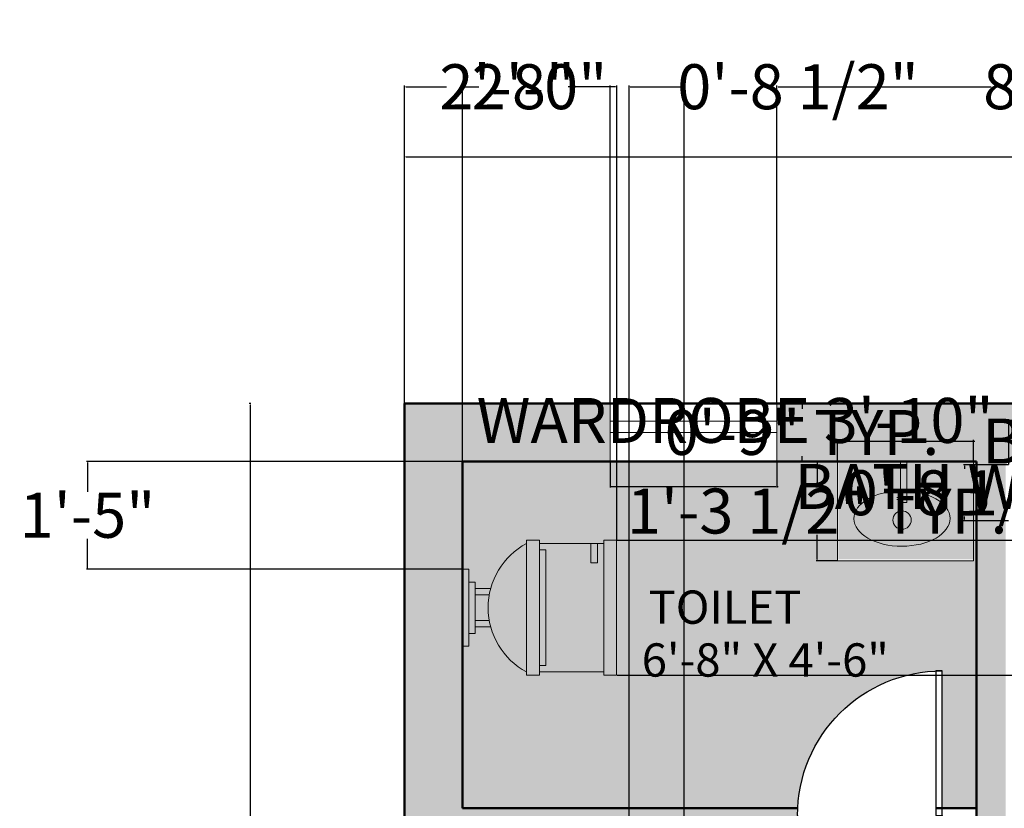
# Model space of a CAD drawing. Units: inches. Extents: x 2974 to 3443, y 2405 to 2963.
# Tile 11 of 13: x 2982 to 3136, y 2840 to 2963. Entities that reach past the tile are written whole.
import ezdxf

# ---------------------------------------------------------------- set-up
doc = ezdxf.new("R2010")
doc.units = ezdxf.units.IN
doc.header["$MEASUREMENT"] = 0
doc.layers.get('0').update_dxf_attribs({"color": 251})
for name, color, linetype, lineweight in [('A-ANNO-DIMS', 2, 'Continuous', 18), ('A-AREA-IDEN', 250, 'Continuous', 25), ('A-DOOR', 32, 'Continuous', 25), ('A-FLOR-FIXT', 8, 'Continuous', 20), ('A-FLOR-FIXT-PATT', 254, 'Continuous', 13), ('A-FLOR-PATT', 9, 'Continuous', 13), ('A-WALL-PATT', 252, 'Continuous', 13), ('walls', 250, 'Continuous', 50), ('windows', 159, 'Continuous', 20)]:
    doc.layers.add(name, color=color, linetype=linetype, lineweight=lineweight)
doc.styles.get("Standard").update_dxf_attribs({"font": 'arial.ttf'})
doc.dimstyles.get("Standard").update_dxf_attribs({"dimtxt": 7, "dimasz": 0.18, "dimexe": 0.18, "dimexo": 0.0625, "dimgap": 0.09, "dimtad": 0, "dimtih": 1, "dimtoh": 1, "dimzin": 0, "dimdsep": 46, "dimlunit": 3, "dimtxsty": 'Standard', "dimcen": 0.09, "dimadec": 0, "dimazin": 0, "dimtfac": 1, "dimtofl": 0, "dimtmove": 0, "dimatfit": 3, "dimfxl": 1, "dimtolj": 1, "dimtzin": 0, "dimarcsym": 0})

# ---------------------------------------------------------------- blocks, each defined once
blk = doc.blocks.new('*U2')
for p, q in [((0, 0), (0, -6)), ((40, 0), (40, -6))]:
    blk.add_line(p, q)
blk.add_lwpolyline([(0, 0), (0, 40), (1.75, 40), (1.75, 0)], close=True)
blk.add_arc((0, 0), 40, 0, 90)
blk = doc.blocks.new('*U18')
for p, q in [((-10, 22), (-10, 12)), ((10, 12), (10, 22)), ((-10, 21), (-7, 21)), ((-7, 20), (-10, 20)), ((-7, 21), (-7, 20)), ((9, 13), (-9, 13)), ((-9, 13), (-9, 12)), ((9, 12), (9, 13)), ((10.5, 12), (-10.5, 12)), ((-10.5, 10), (-10.5, 12)), ((10.5, 12), (10.5, 10)), ((10.5, 10), (-10.5, 10)), ((-3, 4.4065), (-3, 2)), ((-2, 2), (-2, 4.1658)), ((2, 4.1658), (2, 2)), ((3, 2), (3, 4.4065)), ((4, 2), (-4, 2)), ((-4, 2), (-4, 1)), ((4, 1), (4, 2))]:
    blk.add_line(p, q)
for points in [[(10.5, 22), (10.5, 24), (-10.5, 24), (-10.5, 22)], [(6, 0), (6, 1), (-6, 1), (-6, 0)]]:
    blk.add_lwpolyline(points, close=True)
blk.add_arc((0, 15.3333), 11.3333, 208.0725, 331.9275)
blk = doc.blocks.new('*D19')
at = {"layer": 'A-ANNO-DIMS', "color": 0, "lineweight": -2, "transparency": 16777216}
for p, q in [((3042.33, 2937.52), (3042.33, 2941.76)), ((3042.51, 2941.58), (3194.36, 2941.58)), ((3384.15, 2941.58), (3232.3, 2941.58)), ((3384.33, 2937.52), (3384.33, 2941.76))]:
    blk.add_line(p, q, dxfattribs=at)
at = {"layer": 'A-ANNO-DIMS', "color": 0, "transparency": 16777216}
for points in [[(3042.51, 2941.61), (3042.51, 2941.55), (3042.33, 2941.58)], [(3384.15, 2941.61), (3384.15, 2941.55), (3384.33, 2941.58)]]:
    blk.add_solid(points, dxfattribs=at)
at = {"layer": 'Defpoints', "color": 0, "transparency": 16777216}
for p in [(3384.33, 2941.58), (3042.33, 2937.45), (3384.33, 2937.45)]:
    blk.add_point(p, dxfattribs=at)
at = {"layer": 'A-ANNO-DIMS', "color": 0, "transparency": 16777216, "insert": (3213.33, 2941.58), "char_height": 7, "attachment_point": 5}
blk.add_mtext('\\A1;28\'-6.00"', dxfattribs=at)
blk = doc.blocks.new('*D20')
at = {"layer": 'A-ANNO-DIMS', "color": 0, "lineweight": -2, "transparency": 16777216}
for p, q in [((3018.41, 2903.19), (3018.14, 2903.19)), ((3018.32, 2903.01), (3018.32, 2690.85)), ((3018.32, 2471.37), (3018.32, 2683.52)), ((3018.41, 2471.19), (3018.14, 2471.19))]:
    blk.add_line(p, q, dxfattribs=at)
at = {"layer": 'A-ANNO-DIMS', "color": 0, "transparency": 16777216}
for points in [[(3018.29, 2903.01), (3018.35, 2903.01), (3018.32, 2903.19)], [(3018.29, 2471.37), (3018.35, 2471.37), (3018.32, 2471.19)]]:
    blk.add_solid(points, dxfattribs=at)
at = {"layer": 'Defpoints', "color": 0, "transparency": 16777216}
for p in [(3018.47, 2903.19), (3018.32, 2471.19), (3018.47, 2471.19)]:
    blk.add_point(p, dxfattribs=at)
at = {"layer": 'A-ANNO-DIMS', "color": 0, "transparency": 16777216, "insert": (3018.32, 2687.19), "char_height": 7, "attachment_point": 5}
blk.add_mtext("\\A1;36'", dxfattribs=at)
blk = doc.blocks.new('WIN-BATH-26IN')
for p, q in [((0, 0), (0, -9)), ((25.96, 0), (0, 0)), ((0, 0), (0, -2.72)), ((25.96, -9), (25.96, 0)), ((0, -2.72), (25.96, -2.72)), ((25.96, -2.72), (25.96, -4.5)), ((25.96, -4.5), (0, -4.5)), ((0, -9), (25.96, -9))]:
    blk.add_line(p, q)
blk = doc.blocks.new('LAVATORY-WITH-TAP')
h = blk.add_hatch(color=256)
h.dxf.hatch_style = 1
edge = h.paths.add_edge_path()
edge.add_line((0.14, 0.2), (21.04, 0.2))
edge.add_line((21.04, 0.2), (21.04, 15.46))
edge.add_line((21.04, 15.46), (10.75, 15.46))
edge.add_line((10.75, 15.46), (10.75, 10.85))
edge.add_ellipse((10.01, 6.56), major_axis=(-7.48, -0.02), ratio=0.576535, start_angle=272.6137, end_angle=620.1108, ccw=False)
edge.add_line((9.8, 10.87), (9.8, 15.46))
edge.add_line((9.8, 15.46), (0.14, 15.46))
edge.add_line((0.14, 15.46), (0.14, 0.2))
h = blk.add_hatch(color=256)
h.dxf.hatch_style = 1
edge = h.paths.add_edge_path()
edge.add_ellipse((10.01, 6.56), major_axis=(-7.48, -0.02), ratio=0.576535, start_angle=272.6137, end_angle=260.1108)
edge.add_line((10.75, 10.85), (10.75, 9.83))
edge.add_line((10.75, 9.83), (11.35, 9.83))
edge.add_line((11.35, 9.83), (11.35, 9.53))
edge.add_line((11.35, 9.53), (10.75, 9.53))
edge.add_line((10.75, 9.53), (10.75, 9.04))
edge.add_line((10.75, 9.04), (9.8, 9.04))
edge.add_line((9.8, 9.04), (9.8, 10.87))
h.paths.add_polyline_path([(8.24, 6.32, -1), (11.81, 6.32, -1)], flags=16)
h.paths.add_polyline_path([(11.45, 6.32, -1), (8.6, 6.32, -1)], flags=0)
h.paths.add_polyline_path([(8.6, 6.32, 1), (11.45, 6.32, 1)], flags=0)
edge = h.paths.add_edge_path()
edge.add_line((9.8, 9.83), (10.75, 9.83))
edge.add_line((10.75, 9.83), (10.75, 10.85))
edge.add_ellipse((10.01, 6.56), major_axis=(-7.48, -0.02), ratio=0.576535, start_angle=260.1108, end_angle=272.6137)
edge.add_line((9.8, 10.87), (9.8, 9.83))
h.paths.add_polyline_path([(9.8, 9.04), (10.75, 9.04), (10.75, 9.53), (9.8, 9.53)], flags=17)
h.paths.add_polyline_path([(9.8, 9.53), (10.75, 9.53), (10.75, 9.83), (9.8, 9.83)], flags=17)
h.paths.add_polyline_path([(10.75, 9.53), (11.35, 9.53), (11.35, 9.83), (10.75, 9.83)], flags=17)
edge = h.paths.add_edge_path()
edge.add_ellipse((10.01, 6.56), major_axis=(-7.48, -0.02), ratio=0.576535, start_angle=260.1108, end_angle=272.6137, ccw=False)
edge.add_line((10.75, 10.85), (10.75, 15.46))
edge.add_line((10.75, 15.46), (9.8, 15.46))
edge.add_line((9.8, 15.46), (9.8, 10.87))
h = blk.add_hatch(color=256)
h.dxf.hatch_style = 1
h.paths.add_polyline_path([(11.45, 6.32, 1), (8.6, 6.32, 1)], flags=0)
h.paths.add_polyline_path([(11.81, 6.32, 1), (8.24, 6.32, 1)])
h.paths.add_polyline_path([(11.45, 6.32, -1), (8.6, 6.32, -1)], flags=16)
h = blk.add_hatch(color=256)
h.dxf.hatch_style = 1
h.paths.add_polyline_path([(11.45, 6.32, 1), (8.6, 6.32, 1)])
for p, q in [((0, 15.44), (0, 0)), ((9.8, 9.04), (9.8, 15.46)), ((10.75, 9.04), (10.75, 15.46)), ((21.16, 0), (21.16, 15.46)), ((9.22, 9.83), (11.35, 9.83)), ((11.35, 9.53), (9.22, 9.53)), ((9.8, 9.04), (10.75, 9.04)), ((0, 0), (21.16, 0))]:
    blk.add_line(p, q)
blk.add_circle((10.02, 6.32), 1.43)
blk.add_ellipse((10.01, 6.56), major_axis=(-7.48, -0.02), ratio=0.576535)
blk = doc.blocks.new('*D25')
at = {"layer": 'A-ANNO-DIMS', "color": 0, "lineweight": -2, "transparency": 16777216}
for p, q in [((3136.34, 2900.56), (3136.16, 2900.56)), ((3136.34, 2893.72), (3136.34, 2900.74)), ((3182.19, 2900.56), (3136.52, 2900.56)), ((3182.37, 2893.72), (3182.37, 2900.74))]:
    blk.add_line(p, q, dxfattribs=at)
at = {"layer": 'A-ANNO-DIMS', "color": 0, "transparency": 16777216}
for points in [[(3136.52, 2900.59), (3136.52, 2900.53), (3136.34, 2900.56)], [(3182.19, 2900.59), (3182.19, 2900.53), (3182.37, 2900.56)]]:
    blk.add_solid(points, dxfattribs=at)
at = {"layer": 'Defpoints', "color": 0, "transparency": 16777216}
for p in [(3136.34, 2900.56), (3136.34, 2893.66), (3182.37, 2893.66)]:
    blk.add_point(p, dxfattribs=at)
at = {"layer": 'A-ANNO-DIMS', "color": 0, "transparency": 16777216, "insert": (3093.75, 2900.56), "char_height": 7, "attachment_point": 5}
blk.add_mtext('\\A1;WARDROBE 3\'-10"', dxfattribs=at)
blk = doc.blocks.new('*D26')
at = {"layer": 'A-ANNO-DIMS', "color": 0, "lineweight": -2, "transparency": 16777216}
for p, q in [((3136.28, 2893.66), (3129.26, 2893.66)), ((3129.44, 2893.48), (3129.44, 2893.01)), ((3129.44, 2885.13), (3129.44, 2885.59)), ((3136.28, 2884.95), (3129.26, 2884.95))]:
    blk.add_line(p, q, dxfattribs=at)
at = {"layer": 'A-ANNO-DIMS', "color": 0, "transparency": 16777216}
for points in [[(3129.41, 2893.48), (3129.47, 2893.48), (3129.44, 2893.66)], [(3129.41, 2885.13), (3129.47, 2885.13), (3129.44, 2884.95)]]:
    blk.add_solid(points, dxfattribs=at)
at = {"layer": 'Defpoints', "color": 0, "transparency": 16777216}
for p in [(3136.34, 2893.66), (3129.44, 2884.95), (3136.34, 2884.95)]:
    blk.add_point(p, dxfattribs=at)
at = {"layer": 'A-ANNO-DIMS', "color": 0, "transparency": 16777216, "insert": (3129.44, 2889.3), "char_height": 7, "attachment_point": 5}
blk.add_mtext('\\A1;0\'-8 1/2"', dxfattribs=at)
blk = doc.blocks.new('*D28')
at = {"layer": 'A-ANNO-DIMS', "color": 0, "lineweight": -2, "transparency": 16777216}
for p, q in [((3111.77, 2835.69), (3120.92, 2835.69)), ((3120.74, 2835.51), (3120.74, 2833.71)), ((3120.74, 2824.49), (3120.74, 2826.29)), ((3111.77, 2824.31), (3120.92, 2824.31))]:
    blk.add_line(p, q, dxfattribs=at)
at = {"layer": 'A-ANNO-DIMS', "color": 0, "transparency": 16777216}
for points in [[(3120.71, 2835.51), (3120.77, 2835.51), (3120.74, 2835.69)], [(3120.71, 2824.49), (3120.77, 2824.49), (3120.74, 2824.31)]]:
    blk.add_solid(points, dxfattribs=at)
at = {"layer": 'Defpoints', "color": 0, "transparency": 16777216}
for p in [(3111.71, 2835.69), (3111.71, 2824.31), (3120.74, 2824.31)]:
    blk.add_point(p, dxfattribs=at)
at = {"layer": 'A-ANNO-DIMS', "color": 0, "transparency": 16777216, "insert": (3120.74, 2830), "char_height": 7, "attachment_point": 5}
blk.add_mtext('\\A1;0\'-11 1/2"', dxfattribs=at)
blk = doc.blocks.new('*D37')
at = {"layer": 'A-ANNO-DIMS', "color": 0, "lineweight": -2, "transparency": 16777216}
for p, q in [((3074.3, 2894.13), (3074.3, 2890.11)), ((3100.26, 2894.13), (3100.26, 2890.11)), ((3074.48, 2890.29), (3100.08, 2890.29)), ((3100.26, 2890.29), (3100.44, 2890.29))]:
    blk.add_line(p, q, dxfattribs=at)
at = {"layer": 'A-ANNO-DIMS', "color": 0, "transparency": 16777216}
for points in [[(3074.48, 2890.32), (3074.48, 2890.26), (3074.3, 2890.29)], [(3100.08, 2890.32), (3100.08, 2890.26), (3100.26, 2890.29)]]:
    blk.add_solid(points, dxfattribs=at)
at = {"layer": 'Defpoints', "color": 0, "transparency": 16777216}
for p in [(3074.3, 2894.19), (3100.26, 2894.19), (3100.26, 2890.29)]:
    blk.add_point(p, dxfattribs=at)
at = {"layer": 'A-ANNO-DIMS', "color": 0, "transparency": 16777216, "insert": (3158.92, 2890.29), "char_height": 7, "attachment_point": 5}
blk.add_mtext('\\A1;BATH WINDOW 2\'-2" TYP.', dxfattribs=at)
blk = doc.blocks.new('*D38')
at = {"layer": 'A-ANNO-DIMS', "color": 0, "lineweight": -2, "transparency": 16777216}
for p, q in [((3100.33, 2903.19), (3104.34, 2903.19)), ((3104.16, 2903.01), (3104.16, 2902.35)), ((3104.16, 2894.37), (3104.16, 2895.02)), ((3100.33, 2894.19), (3104.34, 2894.19))]:
    blk.add_line(p, q, dxfattribs=at)
at = {"layer": 'A-ANNO-DIMS', "color": 0, "transparency": 16777216}
for points in [[(3104.13, 2903.01), (3104.19, 2903.01), (3104.16, 2903.19)], [(3104.13, 2894.37), (3104.19, 2894.37), (3104.16, 2894.19)]]:
    blk.add_solid(points, dxfattribs=at)
at = {"layer": 'Defpoints', "color": 0, "transparency": 16777216}
for p in [(3100.26, 2903.19), (3104.16, 2903.19), (3100.26, 2894.19)]:
    blk.add_point(p, dxfattribs=at)
at = {"layer": 'A-ANNO-DIMS', "color": 0, "transparency": 16777216, "insert": (3104.16, 2898.69), "char_height": 7, "attachment_point": 5}
blk.add_mtext('\\A1;0\'-9" TYP.', dxfattribs=at)
blk = doc.blocks.new('*D41')
at = {"layer": 'A-ANNO-DIMS', "color": 0, "lineweight": -2, "transparency": 16777216}
for p, q in [((3109.7, 2894.25), (3109.7, 2897.54)), ((3109.88, 2897.36), (3130.68, 2897.36)), ((3130.86, 2894.25), (3130.86, 2897.54)), ((3130.86, 2897.36), (3131.04, 2897.36))]:
    blk.add_line(p, q, dxfattribs=at)
at = {"layer": 'A-ANNO-DIMS', "color": 0, "transparency": 16777216}
for points in [[(3109.88, 2897.39), (3109.88, 2897.33), (3109.7, 2897.36)], [(3130.68, 2897.39), (3130.68, 2897.33), (3130.86, 2897.36)]]:
    blk.add_solid(points, dxfattribs=at)
at = {"layer": 'Defpoints', "color": 0, "transparency": 16777216}
for p in [(3130.86, 2897.36), (3109.7, 2894.19), (3130.86, 2894.19)]:
    blk.add_point(p, dxfattribs=at)
at = {"layer": 'A-ANNO-DIMS', "color": 0, "transparency": 16777216, "insert": (3168.34, 2897.36), "char_height": 7, "attachment_point": 5}
blk.add_mtext('\\A1;BASIN 1\'-9" TYP.', dxfattribs=at)
blk = doc.blocks.new('*D42')
at = {"layer": 'A-ANNO-DIMS', "color": 0, "lineweight": -2, "transparency": 16777216}
for p, q in [((3109.63, 2894.19), (3106.34, 2894.19)), ((3106.52, 2894.01), (3106.52, 2890.17)), ((3106.52, 2878.91), (3106.52, 2882.75)), ((3109.63, 2878.73), (3106.34, 2878.73))]:
    blk.add_line(p, q, dxfattribs=at)
at = {"layer": 'A-ANNO-DIMS', "color": 0, "transparency": 16777216}
for points in [[(3106.49, 2894.01), (3106.55, 2894.01), (3106.52, 2894.19)], [(3106.49, 2878.91), (3106.55, 2878.91), (3106.52, 2878.73)]]:
    blk.add_solid(points, dxfattribs=at)
at = {"layer": 'Defpoints', "color": 0, "transparency": 16777216}
for p in [(3106.52, 2894.19), (3109.7, 2894.19), (3109.7, 2878.73)]:
    blk.add_point(p, dxfattribs=at)
at = {"layer": 'A-ANNO-DIMS', "color": 0, "transparency": 16777216, "insert": (3106.52, 2886.46), "char_height": 7, "attachment_point": 5}
blk.add_mtext('\\A1;1\'-3 1/2" TYP.', dxfattribs=at)
blk = doc.blocks.new('*D51')
at = {"layer": 'A-ANNO-DIMS', "color": 0, "lineweight": -2, "transparency": 16777216}
for p, q in [((3042.33, 2903.25), (3042.33, 2952.68)), ((3042.51, 2952.5), (3048.86, 2952.5)), ((3074.12, 2952.5), (3067.77, 2952.5)), ((3074.3, 2903.25), (3074.3, 2952.68))]:
    blk.add_line(p, q, dxfattribs=at)
at = {"layer": 'A-ANNO-DIMS', "color": 0, "transparency": 16777216}
for points in [[(3042.51, 2952.53), (3042.51, 2952.47), (3042.33, 2952.5)], [(3074.12, 2952.53), (3074.12, 2952.47), (3074.3, 2952.5)]]:
    blk.add_solid(points, dxfattribs=at)
at = {"layer": 'Defpoints', "color": 0, "transparency": 16777216}
for p in [(3074.3, 2952.5), (3042.33, 2903.19), (3074.3, 2903.19)]:
    blk.add_point(p, dxfattribs=at)
at = {"layer": 'A-ANNO-DIMS', "color": 0, "transparency": 16777216, "insert": (3058.31, 2952.5), "char_height": 7, "attachment_point": 5}
blk.add_mtext('\\A1;2\'-8"', dxfattribs=at)
blk = doc.blocks.new('*D52')
at = {"layer": 'A-ANNO-DIMS', "color": 0, "lineweight": -2, "transparency": 16777216}
for p, q in [((3100.26, 2903.25), (3100.26, 2952.68)), ((3100.44, 2952.5), (3133.57, 2952.5)), ((3201.81, 2952.5), (3168.68, 2952.5)), ((3201.99, 2903.25), (3201.99, 2952.68))]:
    blk.add_line(p, q, dxfattribs=at)
at = {"layer": 'A-ANNO-DIMS', "color": 0, "transparency": 16777216}
for points in [[(3100.44, 2952.53), (3100.44, 2952.47), (3100.26, 2952.5)], [(3201.81, 2952.53), (3201.81, 2952.47), (3201.99, 2952.5)]]:
    blk.add_solid(points, dxfattribs=at)
at = {"layer": 'Defpoints', "color": 0, "transparency": 16777216}
for p in [(3201.99, 2952.5), (3100.26, 2903.19), (3201.99, 2903.19)]:
    blk.add_point(p, dxfattribs=at)
at = {"layer": 'A-ANNO-DIMS', "color": 0, "transparency": 16777216, "insert": (3151.13, 2952.5), "char_height": 7, "attachment_point": 5}
blk.add_mtext('\\A1;8\'-5 1/2"', dxfattribs=at)
blk = doc.blocks.new('*D68')
at = {"layer": 'A-ANNO-DIMS', "color": 0, "lineweight": -2, "transparency": 16777216}
for p, q in [((3077.27, 2480.25), (3077.27, 2952.68)), ((3077.45, 2952.5), (3085.63, 2952.5)), ((3085.81, 2480.25), (3085.81, 2952.68)), ((3085.81, 2952.5), (3085.99, 2952.5))]:
    blk.add_line(p, q, dxfattribs=at)
at = {"layer": 'A-ANNO-DIMS', "color": 0, "transparency": 16777216}
for points in [[(3077.45, 2952.53), (3077.45, 2952.47), (3077.27, 2952.5)], [(3085.63, 2952.53), (3085.63, 2952.47), (3085.81, 2952.5)]]:
    blk.add_solid(points, dxfattribs=at)
at = {"layer": 'Defpoints', "color": 0, "transparency": 16777216}
for p in [(3085.81, 2952.5), (3077.27, 2480.19), (3085.81, 2480.19)]:
    blk.add_point(p, dxfattribs=at)
at = {"layer": 'A-ANNO-DIMS', "color": 0, "transparency": 16777216, "insert": (3103.54, 2952.5), "char_height": 7, "attachment_point": 5}
blk.add_mtext('\\A1;0\'-8 1/2"', dxfattribs=at)
blk = doc.blocks.new('*D69')
at = {"layer": 'A-ANNO-DIMS', "color": 0, "lineweight": -2, "transparency": 16777216}
for p, q in [((3051.33, 2877.47), (3051.33, 2952.68)), ((3051.51, 2952.5), (3053.87, 2952.5)), ((3075.15, 2952.5), (3072.78, 2952.5)), ((3075.33, 2881.97), (3075.33, 2952.68))]:
    blk.add_line(p, q, dxfattribs=at)
at = {"layer": 'A-ANNO-DIMS', "color": 0, "transparency": 16777216}
for points in [[(3051.51, 2952.53), (3051.51, 2952.47), (3051.33, 2952.5)], [(3075.15, 2952.53), (3075.15, 2952.47), (3075.33, 2952.5)]]:
    blk.add_solid(points, dxfattribs=at)
at = {"layer": 'Defpoints', "color": 0, "transparency": 16777216}
for p in [(3075.33, 2952.5), (3075.33, 2881.91), (3051.33, 2877.41)]:
    blk.add_point(p, dxfattribs=at)
at = {"layer": 'A-ANNO-DIMS', "color": 0, "transparency": 16777216, "insert": (3063.33, 2952.5), "char_height": 7, "attachment_point": 5}
blk.add_mtext('\\A1;2\'-0"', dxfattribs=at)
blk = doc.blocks.new('*D70')
at = {"layer": 'A-ANNO-DIMS', "color": 0, "lineweight": -2, "transparency": 16777216}
for p, q in [((3075.39, 2881.91), (3409.82, 2881.91)), ((3409.64, 2881.73), (3409.64, 2875.08)), ((3409.64, 2861.09), (3409.64, 2867.75)), ((3075.39, 2860.91), (3409.82, 2860.91))]:
    blk.add_line(p, q, dxfattribs=at)
at = {"layer": 'A-ANNO-DIMS', "color": 0, "transparency": 16777216}
for points in [[(3409.61, 2881.73), (3409.67, 2881.73), (3409.64, 2881.91)], [(3409.61, 2861.09), (3409.67, 2861.09), (3409.64, 2860.91)]]:
    blk.add_solid(points, dxfattribs=at)
at = {"layer": 'Defpoints', "color": 0, "transparency": 16777216}
for p in [(3075.33, 2881.91), (3409.64, 2881.91), (3075.33, 2860.91)]:
    blk.add_point(p, dxfattribs=at)
at = {"layer": 'A-ANNO-DIMS', "color": 0, "transparency": 16777216, "insert": (3409.64, 2871.41), "char_height": 7, "attachment_point": 5}
blk.add_mtext('\\A1;1\'-9"', dxfattribs=at)
blk = doc.blocks.new('*D74')
at = {"layer": 'A-ANNO-DIMS', "color": 0, "lineweight": -2, "transparency": 16777216}
for p, q in [((3051.26, 2894.19), (2992.84, 2894.19)), ((2993.02, 2894.01), (2993.02, 2889.46)), ((2993.02, 2877.59), (2993.02, 2882.14)), ((3051.26, 2877.41), (2992.84, 2877.41))]:
    blk.add_line(p, q, dxfattribs=at)
at = {"layer": 'A-ANNO-DIMS', "color": 0, "transparency": 16777216}
for points in [[(2992.99, 2894.01), (2993.05, 2894.01), (2993.02, 2894.19)], [(2992.99, 2877.59), (2993.05, 2877.59), (2993.02, 2877.41)]]:
    blk.add_solid(points, dxfattribs=at)
at = {"layer": 'Defpoints', "color": 0, "transparency": 16777216}
for p in [(3051.33, 2894.19), (2993.02, 2877.41), (3051.33, 2877.41)]:
    blk.add_point(p, dxfattribs=at)
at = {"layer": 'A-ANNO-DIMS', "color": 0, "transparency": 16777216, "insert": (2993.02, 2885.8), "char_height": 7, "attachment_point": 5}
blk.add_mtext('\\A1;1\'-5"', dxfattribs=at)

msp = doc.modelspace()

# ---------------------------------------------------------------- hatches: boundary and pattern name
at = {"layer": 'A-FLOR-FIXT-PATT'}
h = msp.add_hatch(color=256, dxfattribs=at)
h.dxf.hatch_style = 1
h.paths.add_polyline_path([(3073.326, 2861.412), (3073.326, 2881.412), (3072.326, 2881.412), (3072.326, 2878.412), (3071.326, 2878.412), (3071.326, 2881.412), (3063.326, 2881.412), (3063.326, 2880.412), (3064.326, 2880.412), (3064.326, 2862.412), (3063.326, 2862.412), (3063.326, 2861.412)])
h.paths.add_polyline_path([(3075.326, 2860.912), (3075.326, 2881.912), (3073.326, 2881.912), (3073.326, 2860.912)])
h.paths.add_polyline_path([(3064.326, 2862.412), (3064.326, 2880.412), (3063.326, 2880.412), (3063.326, 2862.412)], flags=17)
h.paths.add_polyline_path([(3063.326, 2860.912), (3063.326, 2881.912), (3061.326, 2881.912), (3061.326, 2860.912)])
h.paths.add_polyline_path([(3061.326, 2861.412), (3061.326, 2881.412, 0.6000022)])
h.paths.add_polyline_path([(3055.504, 2869.412, -0.0889332), (3055.504, 2873.412), (3053.326, 2873.412), (3053.326, 2869.412)])
h.paths.add_polyline_path([(3055.504, 2873.412, -0.0226287), (3055.73, 2874.412), (3053.326, 2874.412), (3053.326, 2873.412)])
h.paths.add_polyline_path([(3055.73, 2868.412, -0.0226287), (3055.504, 2869.412), (3053.326, 2869.412), (3053.326, 2868.412)])
h.paths.add_polyline_path([(3053.326, 2867.412), (3053.326, 2875.412), (3052.326, 2875.412), (3052.326, 2867.412)])
h.paths.add_polyline_path([(3052.326, 2865.412), (3052.326, 2877.412), (3051.326, 2877.412), (3051.326, 2865.412)])
h.paths.add_polyline_path([(3072.326, 2878.412), (3072.326, 2881.412), (3071.326, 2881.412), (3071.326, 2878.412)], flags=17)
at = {"layer": 'A-FLOR-PATT'}
h = msp.add_hatch(dxfattribs=at)
h.set_pattern_fill('ANGLE', color=256, scale=10)
h.set_pattern_definition([(0, (0, 0), (0, 2.75), [2, -0.75]), (90, (0, 0), (-2.75, 2e-16), [2, -0.75])])
h.paths.add_polyline_path([(3240.326, 2894.188), (3220.453, 2894.188), (3220.453, 2893.188), (3218.453, 2893.188), (3218.453, 2892.188), (3217.453, 2892.188), (3217.453, 2889.784, -0.206081), (3224.453, 2884.188), (3224.953, 2884.188), (3224.953, 2882.188), (3224.453, 2882.188), (3224.453, 2872.188), (3224.953, 2872.188), (3224.953, 2870.188), (3203.953, 2870.188), (3203.953, 2872.188), (3204.453, 2872.188), (3204.453, 2882.188), (3203.953, 2882.188), (3203.953, 2884.188), (3204.453, 2884.188, -0.206081), (3211.453, 2889.784), (3211.453, 2892.188), (3210.453, 2892.188), (3210.453, 2893.188), (3208.453, 2893.188), (3208.453, 2894.188), (3201.987, 2894.188), (3188.326, 2894.188), (3188.326, 2835.37), (3203.783, 2835.37), (3203.783, 2814.209), (3188.326, 2814.209), (3188.326, 2808.188), (3215.45, 2808.188, -0.3870418), (3236.952, 2829.559), (3236.952, 2829.581), (3237.937, 2829.581), (3237.937, 2808.188), (3240.326, 2808.188)])
h.paths.add_polyline_path([(3131.326, 2894.188), (3130.856, 2894.188), (3130.856, 2878.731), (3109.695, 2878.731), (3109.695, 2894.188), (3051.326, 2894.188), (3051.326, 2877.412), (3052.326, 2877.412), (3052.326, 2875.412), (3053.326, 2875.412), (3053.326, 2874.412), (3055.73, 2874.412, -0.206081), (3061.326, 2881.412), (3061.326, 2881.912), (3063.326, 2881.912), (3063.326, 2881.412), (3073.326, 2881.412), (3073.326, 2881.912), (3075.326, 2881.912), (3075.326, 2860.912), (3073.326, 2860.912), (3073.326, 2861.412), (3063.326, 2861.412), (3063.326, 2860.912), (3061.326, 2860.912), (3061.326, 2861.412, -0.206081), (3055.73, 2868.412), (3053.326, 2868.412), (3053.326, 2867.412), (3052.326, 2867.412), (3052.326, 2865.412), (3051.326, 2865.412), (3051.326, 2840.188), (3103.485, 2840.188, -0.3870418), (3124.986, 2861.559), (3124.986, 2861.581), (3125.971, 2861.581), (3125.971, 2840.188), (3131.326, 2840.188)])
at = {"layer": 'A-WALL-PATT'}
h = msp.add_hatch(color=256, dxfattribs=at)
h.dxf.hatch_style = 1
h.paths.add_polyline_path([(3222.294, 2555.188), (3211.826, 2555.188), (3211.826, 2657.938), (3207.326, 2657.938), (3207.326, 2555.188), (3051.326, 2555.188), (3051.326, 2583.943), (3042.326, 2583.943), (3042.326, 2471.188), (3165.027, 2471.188), (3165.027, 2480.188), (3051.326, 2480.188), (3051.326, 2550.688), (3222.294, 2550.688)])
h.paths.add_polyline_path([(3188.326, 2700.207), (3183.826, 2700.207), (3183.826, 2691.688), (3051.326, 2691.688), (3051.326, 2740.572), (3042.326, 2740.572), (3042.326, 2651.235), (3045.517, 2651.235), (3051.326, 2651.235), (3051.326, 2687.188), (3188.326, 2687.188)])
h.paths.add_polyline_path([(3051.326, 2894.188), (3074.298, 2894.188), (3074.298, 2903.188), (3042.326, 2903.188), (3042.326, 2807.864), (3045.517, 2807.864), (3051.326, 2807.864), (3051.326, 2835.688), (3103.457, 2835.688), (3103.457, 2839.066, -0.0124729), (3103.485, 2840.188), (3051.326, 2840.188)])
h.paths.add_polyline_path([(3201.987, 2903.188), (3100.263, 2903.188), (3100.263, 2894.188), (3131.326, 2894.188), (3131.326, 2835.688), (3135.826, 2835.688), (3135.826, 2894.188), (3183.826, 2894.188), (3183.826, 2840.188), (3159.826, 2840.188), (3159.826, 2835.688), (3183.826, 2835.688), (3183.826, 2740.207), (3188.326, 2740.207), (3188.326, 2803.688), (3215.422, 2803.688), (3215.422, 2807.066, -0.0124729), (3215.45, 2808.188), (3188.326, 2808.188), (3188.326, 2894.188), (3201.987, 2894.188)])
h.paths.add_polyline_path([(3283.564, 2903.188), (3227.952, 2903.188), (3227.952, 2894.188), (3240.326, 2894.188), (3240.326, 2755.688), (3188.326, 2755.688), (3188.326, 2751.188), (3244.826, 2751.188), (3244.826, 2757.188), (3244.826, 2797.188), (3244.826, 2894.188), (3283.564, 2894.188)])
h.paths.add_polyline_path([(3384.326, 2903.188), (3346.694, 2903.188), (3346.694, 2894.188), (3375.326, 2894.188), (3375.326, 2755.688), (3284.826, 2755.688), (3284.826, 2751.188), (3375.326, 2751.188), (3375.326, 2710.653), (3378.517, 2710.653), (3384.326, 2710.653)])
h.paths.add_polyline_path([(3384.326, 2643.361), (3375.326, 2643.361), (3375.326, 2609.188), (3330.003, 2609.188), (3330.003, 2604.688), (3375.326, 2604.688), (3375.326, 2480.188), (3356.49, 2480.188), (3356.49, 2471.188), (3384.326, 2471.188)])
h.paths.add_polyline_path([(3267.326, 2609.188), (3262.826, 2609.188), (3262.826, 2555.188), (3257.429, 2555.188), (3257.429, 2550.688), (3262.826, 2550.688), (3262.826, 2471.188), (3293.36, 2471.188), (3293.36, 2480.188), (3267.326, 2480.188)])
h.paths.add_polyline_path([(3275.186, 2471.188), (3268.471, 2471.188), (3268.471, 2455.229), (3268.471, 2452.413), (3275.186, 2452.413)])
h.paths.add_polyline_path([(3156.684, 2471.188), (3149.969, 2471.188), (3149.969, 2452.413), (3156.684, 2452.413)])

# ---------------------------------------------------------------- linework, layer by layer
at = {"layer": 'walls'}
for p, q in [((3042.326, 2903.188), (3384.326, 2903.188)), ((3042.326, 2471.188), (3042.326, 2903.188)), ((3051.326, 2894.188), (3131.326, 2894.188)), ((3051.326, 2840.188), (3051.326, 2894.188)), ((3131.326, 2835.688), (3131.326, 2894.188)), ((3051.326, 2840.188), (3103.485, 2840.188)), ((3124.986, 2840.188), (3131.326, 2840.188))]:
    msp.add_line(p, q, dxfattribs=at)

# ---------------------------------------------------------------- block references
at = {"layer": 'A-DOOR', "xscale": -0.5628703588661903, "yscale": 0.5628703588661903, "zscale": 0.5628703588661903}
msp.add_blockref('*U2', (3125.971, 2839.066), dxfattribs=at)
at = {"layer": 'A-FLOR-FIXT'}
msp.add_blockref('LAVATORY-WITH-TAP', (3109.695, 2878.731), dxfattribs=at)
at = {"layer": 'A-FLOR-FIXT', "rotation": 270}
msp.add_blockref('*U18', (3051.326, 2871.412), dxfattribs=at)
at = {"layer": 'windows'}
msp.add_blockref('WIN-BATH-26IN', (3074.298, 2903.188), dxfattribs=at)

# ---------------------------------------------------------------- texts
at = {"layer": 'A-AREA-IDEN'}
for s, height, p in [('TOILET', 5.1811, (3080.287, 2868.909)), ('6\'-8" X 4\'-6"', 5.18112, (3079.227, 2860.687))]:
    msp.add_text(s, height=height, dxfattribs=at).set_placement(p)

# ---------------------------------------------------------------- dimensions: what is measured, and where the dimension line sits
at = {"layer": 'A-ANNO-DIMS'}
for base, p1, p2, override, picture, middle in [((3085.81, 2952.498), (3077.267, 2480.188), (3085.81, 2480.188), {"dimdec": 1, "dimlfac": 1, "dimrnd": 0, "dimzin": 1, "dimdsep": 46, "dimlunit": 4, "dimfrac": 2}, '*D68', (3103.539, 2952.498)), ((3201.987, 2952.498), (3100.263, 2903.188), (3201.987, 2903.188), {"dimdec": 1, "dimlfac": 1, "dimrnd": 0, "dimzin": 1, "dimdsep": 46, "dimlunit": 4, "dimfrac": 2}, '*D52', (3151.125, 2952.498)), ((3074.298, 2952.498), (3042.326, 2903.188), (3074.298, 2903.188), {"dimdec": 1, "dimlfac": 1, "dimrnd": 0, "dimzin": 1, "dimdsep": 46, "dimlunit": 4, "dimfrac": 2}, '*D51', (3058.312, 2952.498)), ((3075.326, 2952.498), (3051.326, 2877.412), (3075.326, 2881.912), {"dimdec": 1, "dimlfac": 1, "dimrnd": 0, "dimzin": 1, "dimdsep": 46, "dimlunit": 4, "dimfrac": 2}, '*D69', (3063.326, 2952.498)), ((3384.326, 2941.584), (3042.326, 2937.454), (3384.326, 2937.454), {"dimclrd": 0, "dimclre": 0, "dimclrt": 0}, '*D19', (3213.326, 2941.584))]:
    dim = msp.add_linear_dim(base=base, p1=p1, p2=p2, dimstyle='Standard', override=override, dxfattribs=at)
    dim.commit()
    dim.dimension.update_dxf_attribs({"geometry": picture, "text_midpoint": middle})
for base, p1, p2, text, picture, middle in [((3130.856, 2897.363), (3109.695, 2894.188), (3130.856, 2894.188), 'BASIN <> TYP.', '*D41', (3168.337, 2897.363)), ((3100.263, 2890.294), (3074.298, 2894.188), (3100.263, 2894.188), 'BATH WINDOW <> TYP.', '*D37', (3158.923, 2890.294))]:
    dim = msp.add_linear_dim(base=base, p1=p1, p2=p2, text=text, dimstyle='Standard', override={"dimdec": 1, "dimlfac": 1, "dimrnd": 0, "dimzin": 1, "dimdsep": 46, "dimlunit": 4, "dimfrac": 2}, dxfattribs=at)
    dim.commit()
    dim.dimension.update_dxf_attribs({"geometry": picture, "text_midpoint": middle})
for base, p1, p2, angle, text, picture, middle in [((3136.34, 2900.56), (3182.368, 2893.656), (3136.34, 2893.656), 180, 'WARDROBE <>', '*D25', (3093.75, 2900.56)), ((3104.158, 2903.188), (3100.263, 2894.188), (3100.263, 2903.188), 90, '<> TYP.', '*D38', (3104.158, 2898.688)), ((3106.521, 2894.188), (3109.695, 2878.731), (3109.695, 2894.188), 90, '<> TYP.', '*D42', (3106.521, 2886.46))]:
    dim = msp.add_linear_dim(base=base, p1=p1, p2=p2, angle=angle, text=text, dimstyle='Standard', override={"dimdec": 1, "dimlfac": 1, "dimrnd": 0, "dimzin": 1, "dimdsep": 46, "dimlunit": 4, "dimfrac": 2}, dxfattribs=at)
    dim.commit()
    dim.dimension.update_dxf_attribs({"geometry": picture, "text_midpoint": middle})
for base, p1, p2, angle, override, picture, middle in [((3018.319, 2471.188), (3018.469, 2903.188), (3018.469, 2471.188), 90, {"dimclrd": 0, "dimclre": 0, "dimclrt": 0}, '*D20', (3018.319, 2687.188)), ((3129.436, 2884.951), (3136.34, 2893.656), (3136.34, 2884.951), 270, {"dimdec": 1, "dimlfac": 1, "dimrnd": 0, "dimzin": 1, "dimdsep": 46, "dimlunit": 4, "dimfrac": 2}, '*D26', (3129.436, 2889.303)), ((2993.016, 2877.412), (3051.326, 2894.188), (3051.326, 2877.412), 90, {"dimdec": 1, "dimlfac": 1, "dimrnd": 0, "dimzin": 1, "dimdsep": 46, "dimlunit": 4, "dimfrac": 2}, '*D74', (2993.016, 2885.8)), ((3409.636, 2881.912), (3075.326, 2860.912), (3075.326, 2881.912), 90, {"dimdec": 1, "dimlfac": 1, "dimrnd": 0, "dimzin": 1, "dimdsep": 46, "dimlunit": 4, "dimfrac": 2}, '*D70', (3409.636, 2871.412)), ((3120.74, 2824.306), (3111.712, 2835.688), (3111.712, 2824.306), 270, {"dimdec": 1, "dimlfac": 1, "dimrnd": 0, "dimzin": 1, "dimdsep": 46, "dimlunit": 4, "dimfrac": 2}, '*D28', (3120.74, 2829.997))]:
    dim = msp.add_linear_dim(base=base, p1=p1, p2=p2, angle=angle, dimstyle='Standard', override=override, dxfattribs=at)
    dim.commit()
    dim.dimension.update_dxf_attribs({"geometry": picture, "text_midpoint": middle})

doc.saveas('drawing.dxf')
